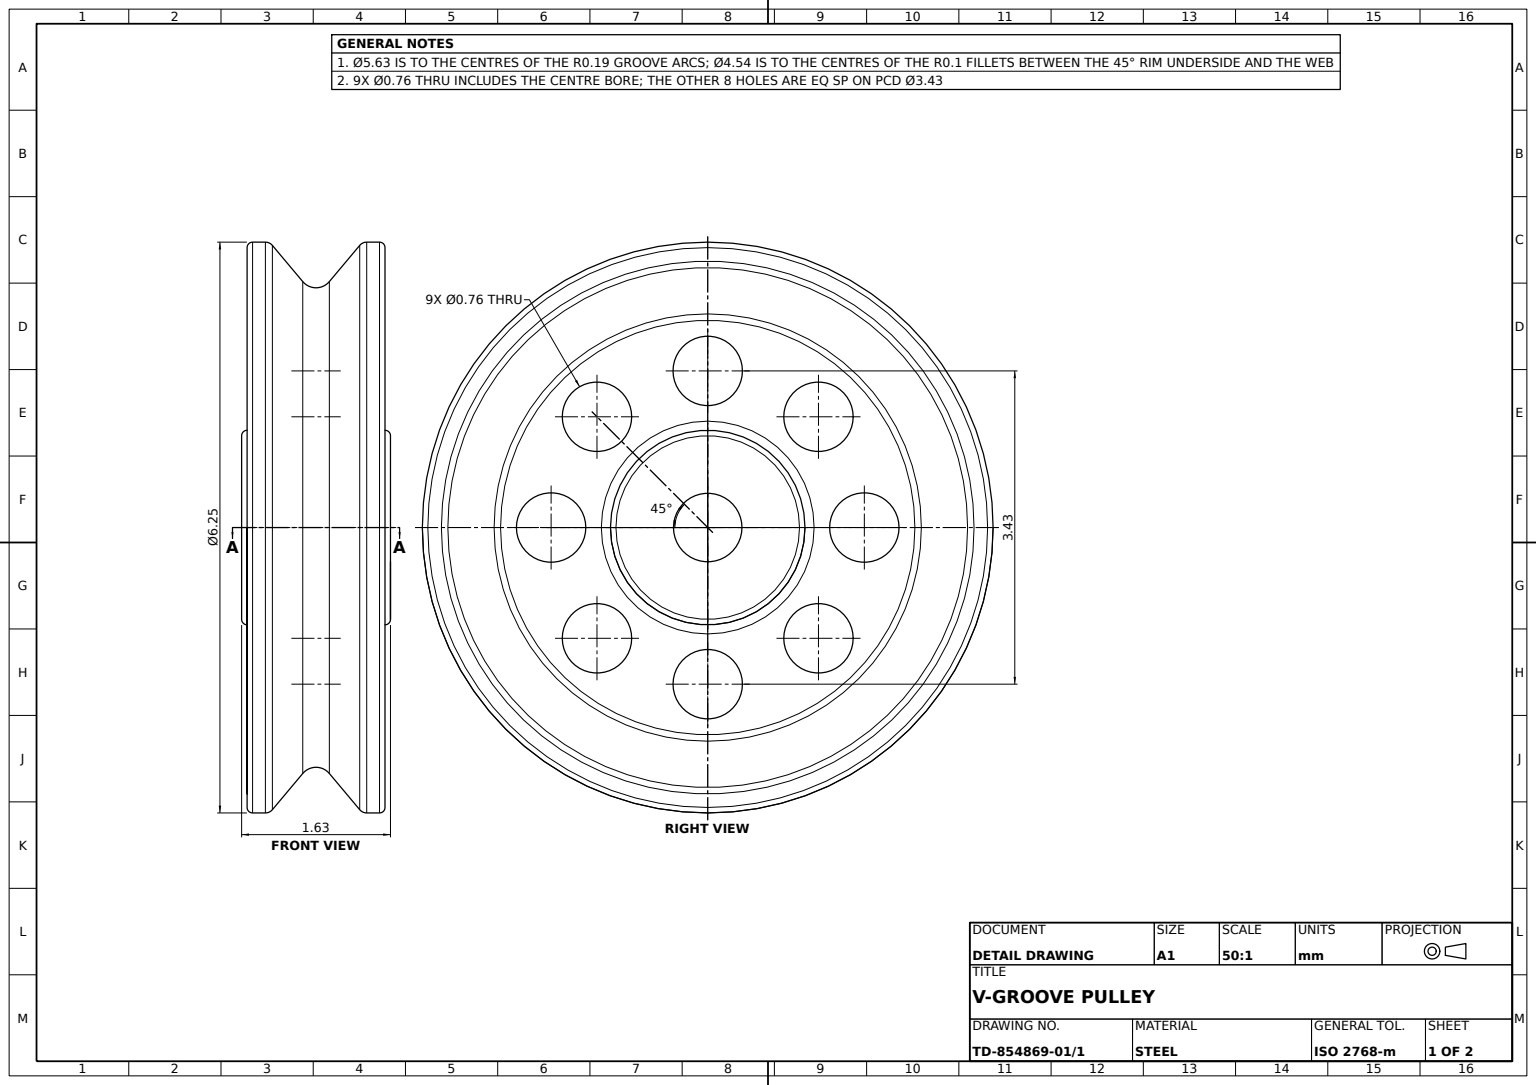
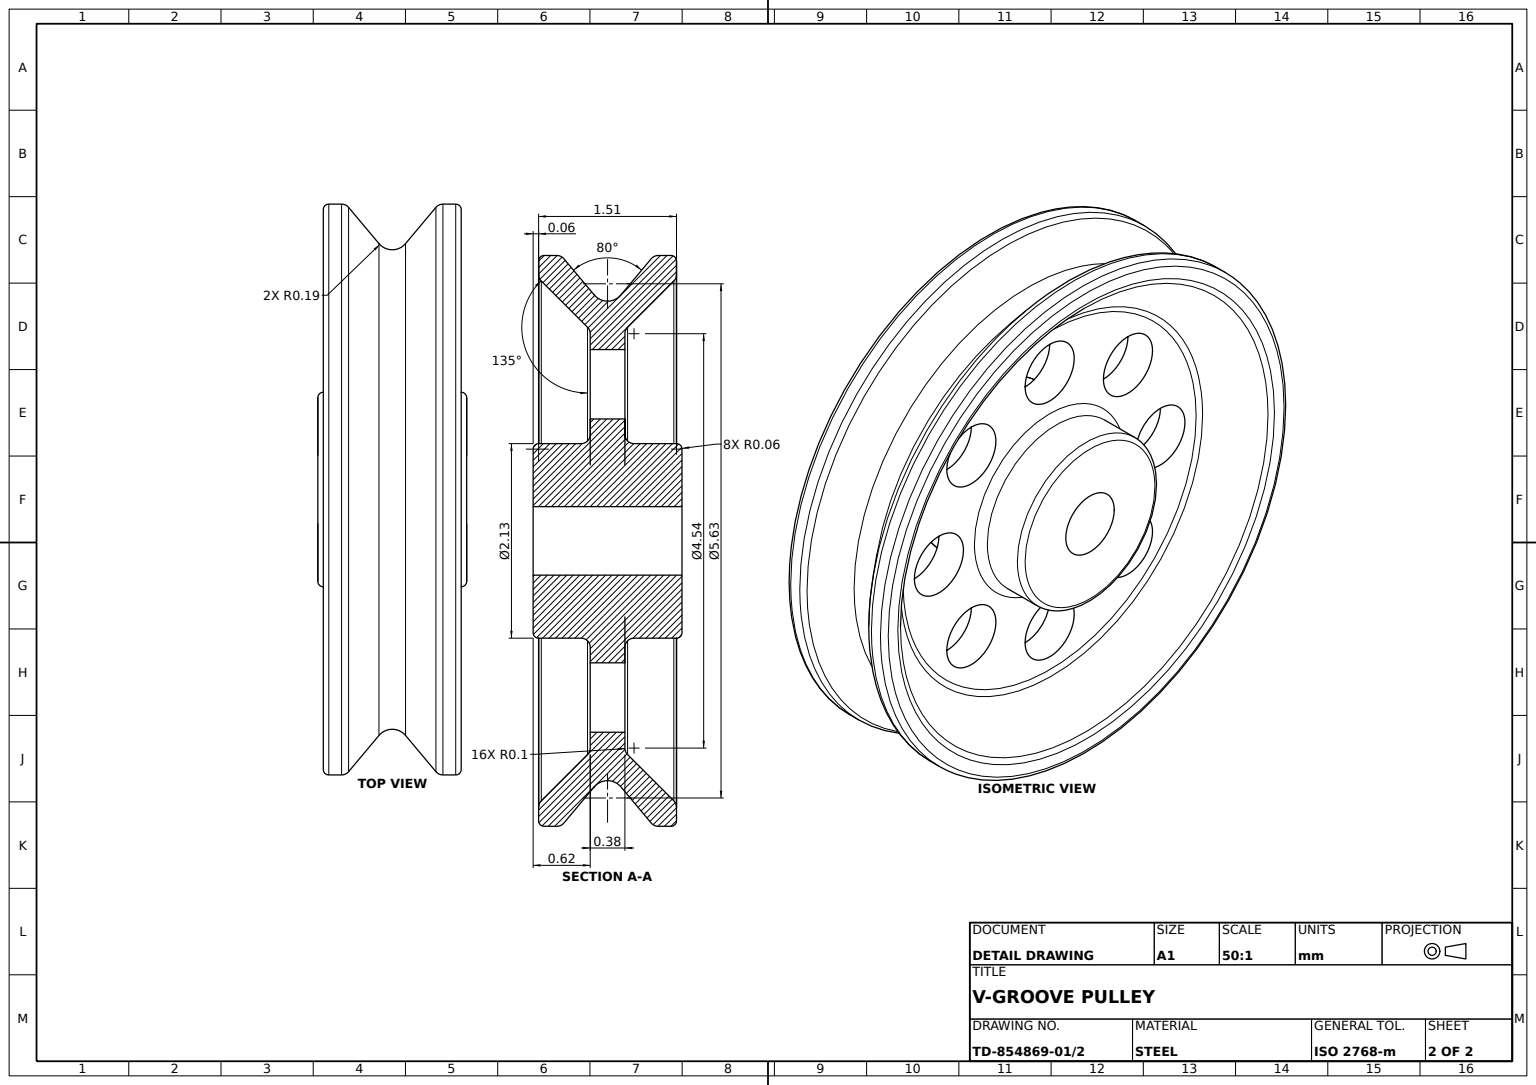
from build123d import *

# Parameters (mm, degrees)
LIGHTENING_HOLES_SKETCH_R      = 0.38
LIGHTENING_HOLES_8X_0_76_DEPTH = 5.532248476


with BuildPart() as part:
    # Pulley Profile Sketch → Pulley Body (revolve)
    with BuildSketch(Plane(origin=(0, 0, 0), x_dir=(0, 0, -1), z_dir=(1, 0, 0)), mode=Mode.PRIVATE) as pulley_body_sk:
        with BuildLine():
            Line((0.815, 0.375), (-0.815, 0.375))
            Line((-0.815, 0.375), (-0.815, 1.005))
            ThreePointArc((-0.815, 1.005), (-0.797426407, 1.047426407), (-0.755, 1.065))
            Line((-0.755, 1.065), (-0.29, 1.065))
            ThreePointArc((-0.29, 1.065), (-0.219289322, 1.094289322), (-0.19, 1.165))
            Line((-0.19, 1.165), (-0.19, 2.268578644))
            ThreePointArc((-0.19, 2.268578644), (-0.197612047, 2.306846987), (-0.219289322, 2.339289322))
            Line((-0.219289322, 2.339289322), (-0.725710678, 2.845710678))
            ThreePointArc((-0.725710678, 2.845710678), (-0.747387953, 2.878153013), (-0.755, 2.916421356))
            Line((-0.755, 2.916421356), (-0.755, 3.065))
            ThreePointArc((-0.755, 3.065), (-0.737426407, 3.107426407), (-0.695, 3.125))
            Line((-0.695, 3.125), (-0.554779036, 3.125))
            ThreePointArc((-0.554779036, 3.125), (-0.51251721, 3.115630779), (-0.478174592, 3.089278761))
            Line((-0.478174592, 3.089278761), (-0.145548444, 2.692870354))
            ThreePointArc((-0.145548444, 2.692870354), (0, 2.625), (0.145548444, 2.692870354))
            Line((0.145548444, 2.692870354), (0.478174592, 3.089278761))
            ThreePointArc((0.478174592, 3.089278761), (0.51251721, 3.115630779), (0.554779036, 3.125))
            Line((0.554779036, 3.125), (0.695, 3.125))
            ThreePointArc((0.695, 3.125), (0.737426407, 3.107426407), (0.755, 3.065))
            Line((0.755, 3.065), (0.755, 2.916421356))
            ThreePointArc((0.755, 2.916421356), (0.747387953, 2.878153013), (0.725710678, 2.845710678))
            Line((0.725710678, 2.845710678), (0.219289322, 2.339289322))
            ThreePointArc((0.219289322, 2.339289322), (0.197612047, 2.306846987), (0.19, 2.268578644))
            Line((0.19, 2.268578644), (0.19, 1.165))
            ThreePointArc((0.19, 1.165), (0.219289322, 1.094289322), (0.29, 1.065))
            Line((0.29, 1.065), (0.755, 1.065))
            ThreePointArc((0.755, 1.065), (0.797426407, 1.047426407), (0.815, 1.005))
            Line((0.815, 1.005), (0.815, 0.375))
        make_face()
    revolve(pulley_body_sk.sketch.rotate(Axis((0, 0, 29.195986036), (0, 0, -1)), 90), axis=Axis((0, 0, 29.195986036), (0, 0, -1)))

    # Lightening Holes Sketch → Lightening Holes 8xØ0.76 (cut, through all)
    with BuildSketch(Plane.XY.offset(0.19)):
        with Locations((0, 1.715)):
            Circle(LIGHTENING_HOLES_SKETCH_R)
        with Locations((-1.21268813, 1.21268813)):
            Circle(LIGHTENING_HOLES_SKETCH_R)
        with Locations((-1.715, 0)):
            Circle(LIGHTENING_HOLES_SKETCH_R)
        with Locations((-1.21268813, -1.21268813)):
            Circle(LIGHTENING_HOLES_SKETCH_R)
        with Locations((0, -1.715)):
            Circle(LIGHTENING_HOLES_SKETCH_R)
        with Locations((1.21268813, -1.21268813)):
            Circle(LIGHTENING_HOLES_SKETCH_R)
        with Locations((1.715, 0)):
            Circle(LIGHTENING_HOLES_SKETCH_R)
        with Locations((1.21268813, 1.21268813)):
            Circle(LIGHTENING_HOLES_SKETCH_R)
    extrude(amount=-LIGHTENING_HOLES_8X_0_76_DEPTH, mode=Mode.SUBTRACT)


solid = part.part
